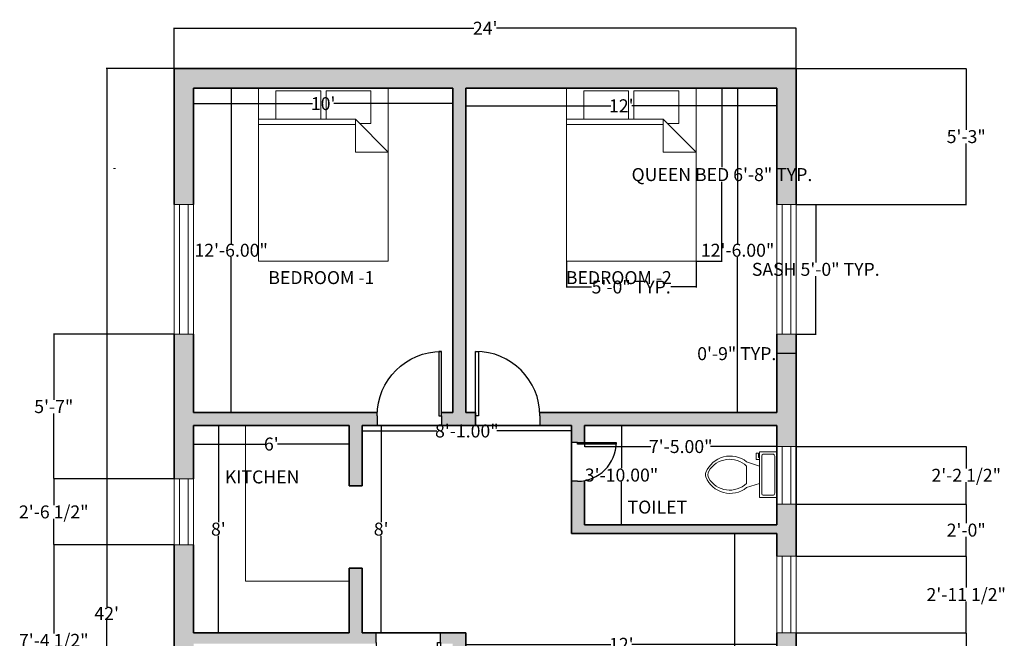
# Model space of a CAD drawing. Units: inches. Extents: x -54 to 402, y -41 to 548.
# Tile 2 of 2: x -53 to 402, y 261 to 548. Entities that reach past the tile are written whole.
import ezdxf

# ---------------------------------------------------------------- set-up
doc = ezdxf.new("R2010")
doc.units = ezdxf.units.IN
doc.header["$MEASUREMENT"] = 0
for name, color, linetype, lineweight in [('A-ANNO-DIMS', 2, 'Continuous', 18), ('A-AREA-IDEN', 7, 'Continuous', 25), ('A-DOOR', 4, 'Continuous', 25), ('A-FLOR-CASE', 8, 'Continuous', 18), ('A-FLOR-FIXT', 9, 'Continuous', 18), ('A-FURN', 8, 'Continuous', 18), ('A-GLAZ', 5, 'Continuous', 18), ('A-REFR', 8, 'Continuous', 13), ('A-WALL', 7, 'Continuous', 35)]:
    doc.layers.add(name, color=color, linetype=linetype, lineweight=lineweight)
doc.layers.add('A-WALL-PATT', color=18, linetype='Continuous', lineweight=13, true_color=0x000000)
doc.styles.get("Standard").update_dxf_attribs({"font": 'arial.ttf'})
doc.dimstyles.get("Standard").update_dxf_attribs({"dimtxt": 6, "dimasz": 0.18, "dimexe": 0.18, "dimexo": 0.0625, "dimgap": 0.09, "dimtad": 0, "dimtih": 1, "dimtoh": 1, "dimzin": 0, "dimdsep": 46, "dimlunit": 3, "dimtxsty": 'Standard', "dimcen": 0.09, "dimadec": 0, "dimazin": 0, "dimtfac": 1, "dimtofl": 0, "dimtmove": 0, "dimatfit": 3, "dimfxl": 1, "dimtolj": 1, "dimtzin": 0, "dimarcsym": 0})

# ---------------------------------------------------------------- blocks, each defined once
blk = doc.blocks.new('*U2')
for p, q in [((0, 0), (0, -6)), ((40, 0), (40, -6))]:
    blk.add_line(p, q)
blk.add_lwpolyline([(0, 0), (0, 40), (1.75, 40), (1.75, 0)], close=True)
blk.add_arc((0, 0), 40, 0, 90)
blk = doc.blocks.new('Bed - Queen')
for p, q in [((0, -80.00003), (0, 0)), ((0, 0), (59.99999, 0)), ((59.99999, 0), (59.99999, -80.00003)), ((7.99999, -1.2), (28.79998, -1.2)), ((7.99999, -14.4), (7.99999, -1.2)), ((28.79998, -1.2), (28.79998, -14.4)), ((31.19999, -1.2), (51.99999, -1.2)), ((31.19999, -14.4), (31.19999, -1.2)), ((51.99999, -1.2), (51.99999, -16.4)), ((0, -14.4), (44.8, -14.4)), ((44.8, -16.8), (0, -16.8)), ((59.99999, -29.6), (44.8, -14.4)), ((44.8, -14.4), (44.8, -29.6)), ((51.99999, -16.4), (46.79936, -16.4)), ((44.8, -29.6), (59.99999, -29.6)), ((59.99999, -80.00003), (0, -80.00003))]:
    blk.add_line(p, q)
blk = doc.blocks.new('*U5')
for p, q in [((9.5, -6), (9.5, -2)), ((-10, -8.5), (-8, -8.5)), ((-10, -9.5), (-10, -8.5)), ((-8, -8.5), (-8, -8)), ((-7, -8), (-7, -9.5)), ((-4, -8), (-6, -14)), ((4, -8), (6, -14)), ((-7, -9.5), (-10, -9.5)), ((4, -14), (-4, -14))]:
    blk.add_line(p, q)
blk.add_lwpolyline([(10.5, -8), (10.5, 0), (-10.5, 0), (-10.5, -8)], close=True)
for points in [[(-9.5, -2), (-9.5, -6)], [(8.5, -1), (-8.5, -1)], [(-8.5, -7), (8.5, -7)]]:
    blk.add_lwpolyline(points)
for centre, radius, start, end in [((-8.62, -1.88), 0.884, 81.8699, 188.1301), ((8.62, -1.88), 0.884, 351.8699, 98.1301), ((-8.62, -6.12), 0.884, 171.8699, 278.1301), ((8.62, -6.12), 0.884, 261.8699, 8.1301), ((3.52, -21.58), 12.17, 141.4691, 247.9714), ((4.2, -21.82), 11.33, 136.3677, 238.9468), ((-3.52, -21.58), 12.17, 292.0284, 38.5307), ((-4.2, -21.82), 11.33, 301.053, 43.6321), ((0, -27.88), 4, 245.7318, 294.2682), ((0, -29), 4, 254.8605, 285.1395)]:
    blk.add_arc(centre, radius, start, end)
blk = doc.blocks.new('*D6')
at = {"layer": 'A-ANNO-DIMS', "color": 0, "lineweight": -2, "transparency": 16777216}
for p, q in [((18.08, 524.92), (18.08, 543.75)), ((18.26, 543.57), (156.84, 543.57)), ((305.9, 543.57), (167.31, 543.57)), ((306.08, 524.92), (306.08, 543.75))]:
    blk.add_line(p, q, dxfattribs=at)
at = {"layer": 'A-ANNO-DIMS', "color": 0, "transparency": 16777216}
for points in [[(18.26, 543.6), (18.26, 543.54), (18.08, 543.57)], [(305.9, 543.6), (305.9, 543.54), (306.08, 543.57)]]:
    blk.add_solid(points, dxfattribs=at)
at = {"layer": 'Defpoints', "color": 0, "transparency": 16777216}
for p in [(306.08, 543.57), (18.08, 524.86), (306.08, 524.86)]:
    blk.add_point(p, dxfattribs=at)
at = {"layer": 'A-ANNO-DIMS', "color": 0, "transparency": 16777216, "insert": (162.08, 543.57), "char_height": 6, "attachment_point": 5}
blk.add_mtext("\\A1;24'", dxfattribs=at)
blk = doc.blocks.new('*D7')
at = {"layer": 'A-ANNO-DIMS', "color": 0, "lineweight": -2, "transparency": 16777216}
for p, q in [((18.01, 524.86), (-13.3, 524.86)), ((-13.12, 524.68), (-13.12, 275.96)), ((-13.12, 21.04), (-13.12, 269.76)), ((18.01, 20.86), (-13.3, 20.86))]:
    blk.add_line(p, q, dxfattribs=at)
at = {"layer": 'A-ANNO-DIMS', "color": 0, "transparency": 16777216}
for points in [[(-13.15, 524.68), (-13.09, 524.68), (-13.12, 524.86)], [(-13.15, 21.04), (-13.09, 21.04), (-13.12, 20.86)]]:
    blk.add_solid(points, dxfattribs=at)
at = {"layer": 'Defpoints', "color": 0, "transparency": 16777216}
for p in [(18.08, 524.86), (-13.12, 20.86), (18.08, 20.86)]:
    blk.add_point(p, dxfattribs=at)
at = {"layer": 'A-ANNO-DIMS', "color": 0, "transparency": 16777216, "insert": (-13.12, 272.86), "char_height": 6, "attachment_point": 5}
blk.add_mtext("\\A1;42'", dxfattribs=at)
blk = doc.blocks.new('*D15')
at = {"layer": 'A-ANNO-DIMS', "color": 0, "lineweight": -2, "transparency": 16777216}
for p, q in [((153.08, 263.8), (153.08, 258.38)), ((297.08, 263.8), (297.08, 258.38)), ((153.26, 258.56), (220.18, 258.56)), ((296.9, 258.56), (229.98, 258.56))]:
    blk.add_line(p, q, dxfattribs=at)
at = {"layer": 'A-ANNO-DIMS', "color": 0, "transparency": 16777216}
for points in [[(153.26, 258.59), (153.26, 258.53), (153.08, 258.56)], [(296.9, 258.59), (296.9, 258.53), (297.08, 258.56)]]:
    blk.add_solid(points, dxfattribs=at)
at = {"layer": 'Defpoints', "color": 0, "transparency": 16777216}
for p in [(153.08, 263.86), (297.08, 263.86), (297.08, 258.56)]:
    blk.add_point(p, dxfattribs=at)
at = {"layer": 'A-ANNO-DIMS', "color": 0, "transparency": 16777216, "insert": (225.08, 258.56), "char_height": 6, "attachment_point": 5}
blk.add_mtext("\\A1;12'", dxfattribs=at)
blk = doc.blocks.new('*D16')
at = {"layer": 'A-ANNO-DIMS', "color": 0, "lineweight": -2, "transparency": 16777216}
for p, q in [((297.01, 309.86), (277.33, 309.86)), ((277.51, 309.68), (277.51, 227.01)), ((277.51, 138.04), (277.51, 220.71)), ((297.01, 137.86), (277.33, 137.86))]:
    blk.add_line(p, q, dxfattribs=at)
at = {"layer": 'A-ANNO-DIMS', "color": 0, "transparency": 16777216}
for points in [[(277.48, 309.68), (277.54, 309.68), (277.51, 309.86)], [(277.48, 138.04), (277.54, 138.04), (277.51, 137.86)]]:
    blk.add_solid(points, dxfattribs=at)
at = {"layer": 'Defpoints', "color": 0, "transparency": 16777216}
for p in [(297.08, 309.86), (277.51, 137.86), (297.08, 137.86)]:
    blk.add_point(p, dxfattribs=at)
at = {"layer": 'A-ANNO-DIMS', "color": 0, "transparency": 16777216, "insert": (277.51, 223.86), "char_height": 6, "attachment_point": 5}
blk.add_mtext('\\A1;14\'-4.00"', dxfattribs=at)
blk = doc.blocks.new('*D17')
at = {"layer": 'A-ANNO-DIMS', "color": 0, "lineweight": -2, "transparency": 16777216}
for p, q in [((27.08, 359.8), (27.08, 351.03)), ((99.08, 359.8), (99.08, 351.03)), ((27.26, 351.21), (60.21, 351.21)), ((98.9, 351.21), (65.94, 351.21))]:
    blk.add_line(p, q, dxfattribs=at)
at = {"layer": 'A-ANNO-DIMS', "color": 0, "transparency": 16777216}
for points in [[(27.26, 351.24), (27.26, 351.18), (27.08, 351.21)], [(98.9, 351.24), (98.9, 351.18), (99.08, 351.21)]]:
    blk.add_solid(points, dxfattribs=at)
at = {"layer": 'Defpoints', "color": 0, "transparency": 16777216}
for p in [(27.08, 359.86), (99.08, 359.86), (99.08, 351.21)]:
    blk.add_point(p, dxfattribs=at)
at = {"layer": 'A-ANNO-DIMS', "color": 0, "transparency": 16777216, "insert": (63.08, 351.21), "char_height": 6, "attachment_point": 5}
blk.add_mtext("\\A1;6'", dxfattribs=at)
blk = doc.blocks.new('*D18')
at = {"layer": 'A-ANNO-DIMS', "color": 0, "lineweight": -2, "transparency": 16777216}
for p, q in [((32.47, 359.86), (38.75, 359.86)), ((38.57, 359.68), (38.57, 315.01)), ((38.57, 264.04), (38.57, 308.71)), ((32.47, 263.86), (38.75, 263.86))]:
    blk.add_line(p, q, dxfattribs=at)
at = {"layer": 'A-ANNO-DIMS', "color": 0, "transparency": 16777216}
for points in [[(38.54, 359.68), (38.6, 359.68), (38.57, 359.86)], [(38.54, 264.04), (38.6, 264.04), (38.57, 263.86)]]:
    blk.add_solid(points, dxfattribs=at)
at = {"layer": 'Defpoints', "color": 0, "transparency": 16777216}
for p in [(32.41, 359.86), (32.41, 263.86), (38.57, 263.86)]:
    blk.add_point(p, dxfattribs=at)
at = {"layer": 'A-ANNO-DIMS', "color": 0, "transparency": 16777216, "insert": (38.57, 311.86), "char_height": 6, "attachment_point": 5}
blk.add_mtext("\\A1;8'", dxfattribs=at)
blk = doc.blocks.new('*D19')
at = {"layer": 'A-ANNO-DIMS', "color": 0, "lineweight": -2, "transparency": 16777216}
for p, q in [((208.14, 359.86), (225.36, 359.86)), ((225.18, 359.68), (225.18, 340.02)), ((225.18, 314.04), (225.18, 333.71)), ((208.14, 313.86), (225.36, 313.86))]:
    blk.add_line(p, q, dxfattribs=at)
at = {"layer": 'A-ANNO-DIMS', "color": 0, "transparency": 16777216}
for points in [[(225.15, 359.68), (225.21, 359.68), (225.18, 359.86)], [(225.15, 314.04), (225.21, 314.04), (225.18, 313.86)]]:
    blk.add_solid(points, dxfattribs=at)
at = {"layer": 'Defpoints', "color": 0, "transparency": 16777216}
for p in [(208.08, 359.86), (208.08, 313.86), (225.18, 313.86)]:
    blk.add_point(p, dxfattribs=at)
at = {"layer": 'A-ANNO-DIMS', "color": 0, "transparency": 16777216, "insert": (225.18, 336.86), "char_height": 6, "attachment_point": 5}
blk.add_mtext('\\A1;3\'-10.00"', dxfattribs=at)
blk = doc.blocks.new('*D20')
at = {"layer": 'A-ANNO-DIMS', "color": 0, "lineweight": -2, "transparency": 16777216}
for p, q in [((208.08, 359.8), (208.08, 349.88)), ((297.08, 359.8), (297.08, 349.88)), ((208.26, 350.06), (238.71, 350.06)), ((296.9, 350.06), (266.44, 350.06))]:
    blk.add_line(p, q, dxfattribs=at)
at = {"layer": 'A-ANNO-DIMS', "color": 0, "transparency": 16777216}
for points in [[(208.26, 350.09), (208.26, 350.03), (208.08, 350.06)], [(296.9, 350.09), (296.9, 350.03), (297.08, 350.06)]]:
    blk.add_solid(points, dxfattribs=at)
at = {"layer": 'Defpoints', "color": 0, "transparency": 16777216}
for p in [(208.08, 359.86), (297.08, 359.86), (297.08, 350.06)]:
    blk.add_point(p, dxfattribs=at)
at = {"layer": 'A-ANNO-DIMS', "color": 0, "transparency": 16777216, "insert": (252.58, 350.06), "char_height": 6, "attachment_point": 5}
blk.add_mtext('\\A1;7\'-5.00"', dxfattribs=at)
blk = doc.blocks.new('*D21')
at = {"layer": 'A-ANNO-DIMS', "color": 0, "lineweight": -2, "transparency": 16777216}
for p, q in [((153.08, 515.8), (153.08, 507.5)), ((297.08, 515.8), (297.08, 507.5)), ((153.26, 507.68), (220.18, 507.68)), ((296.9, 507.68), (229.98, 507.68))]:
    blk.add_line(p, q, dxfattribs=at)
at = {"layer": 'A-ANNO-DIMS', "color": 0, "transparency": 16777216}
for points in [[(153.26, 507.71), (153.26, 507.65), (153.08, 507.68)], [(296.9, 507.71), (296.9, 507.65), (297.08, 507.68)]]:
    blk.add_solid(points, dxfattribs=at)
at = {"layer": 'Defpoints', "color": 0, "transparency": 16777216}
for p in [(153.08, 515.86), (297.08, 515.86), (297.08, 507.68)]:
    blk.add_point(p, dxfattribs=at)
at = {"layer": 'A-ANNO-DIMS', "color": 0, "transparency": 16777216, "insert": (225.08, 507.68), "char_height": 6, "attachment_point": 5}
blk.add_mtext("\\A1;12'", dxfattribs=at)
blk = doc.blocks.new('*D22')
at = {"layer": 'A-ANNO-DIMS', "color": 0, "lineweight": -2, "transparency": 16777216}
for p, q in [((297.01, 515.86), (278.73, 515.86)), ((278.91, 515.68), (278.91, 444.01)), ((278.91, 366.04), (278.91, 437.71)), ((297.01, 365.86), (278.73, 365.86))]:
    blk.add_line(p, q, dxfattribs=at)
at = {"layer": 'A-ANNO-DIMS', "color": 0, "transparency": 16777216}
for points in [[(278.88, 515.68), (278.94, 515.68), (278.91, 515.86)], [(278.88, 366.04), (278.94, 366.04), (278.91, 365.86)]]:
    blk.add_solid(points, dxfattribs=at)
at = {"layer": 'Defpoints', "color": 0, "transparency": 16777216}
for p in [(297.08, 515.86), (278.91, 365.86), (297.08, 365.86)]:
    blk.add_point(p, dxfattribs=at)
at = {"layer": 'A-ANNO-DIMS', "color": 0, "transparency": 16777216, "insert": (278.91, 440.86), "char_height": 6, "attachment_point": 5}
blk.add_mtext('\\A1;12\'-6.00"', dxfattribs=at)
blk = doc.blocks.new('*D23')
at = {"layer": 'A-ANNO-DIMS', "color": 0, "lineweight": -2, "transparency": 16777216}
for p, q in [((27.08, 515.8), (27.08, 508.5)), ((147.08, 515.8), (147.08, 508.5)), ((27.26, 508.68), (82.18, 508.68)), ((146.9, 508.68), (91.98, 508.68))]:
    blk.add_line(p, q, dxfattribs=at)
at = {"layer": 'A-ANNO-DIMS', "color": 0, "transparency": 16777216}
for points in [[(27.26, 508.71), (27.26, 508.65), (27.08, 508.68)], [(146.9, 508.71), (146.9, 508.65), (147.08, 508.68)]]:
    blk.add_solid(points, dxfattribs=at)
at = {"layer": 'Defpoints', "color": 0, "transparency": 16777216}
for p in [(27.08, 515.86), (147.08, 515.86), (147.08, 508.68)]:
    blk.add_point(p, dxfattribs=at)
at = {"layer": 'A-ANNO-DIMS', "color": 0, "transparency": 16777216, "insert": (87.08, 508.68), "char_height": 6, "attachment_point": 5}
blk.add_mtext("\\A1;10'", dxfattribs=at)
blk = doc.blocks.new('*D24')
at = {"layer": 'A-ANNO-DIMS', "color": 0, "lineweight": -2, "transparency": 16777216}
for p, q in [((46.31, 515.86), (44.31, 515.86)), ((44.49, 515.68), (44.49, 444.01)), ((44.49, 366.04), (44.49, 437.71)), ((46.31, 365.86), (44.31, 365.86))]:
    blk.add_line(p, q, dxfattribs=at)
at = {"layer": 'A-ANNO-DIMS', "color": 0, "transparency": 16777216}
for points in [[(44.46, 515.68), (44.52, 515.68), (44.49, 515.86)], [(44.46, 366.04), (44.52, 366.04), (44.49, 365.86)]]:
    blk.add_solid(points, dxfattribs=at)
at = {"layer": 'Defpoints', "color": 0, "transparency": 16777216}
for p in [(46.37, 515.86), (44.49, 365.86), (46.37, 365.86)]:
    blk.add_point(p, dxfattribs=at)
at = {"layer": 'A-ANNO-DIMS', "color": 0, "transparency": 16777216, "insert": (44.49, 440.86), "char_height": 6, "attachment_point": 5}
blk.add_mtext('\\A1;12\'-6.00"', dxfattribs=at)
blk = doc.blocks.new('*D25')
at = {"layer": 'A-ANNO-DIMS', "color": 0, "lineweight": -2, "transparency": 16777216}
for p, q in [((105.08, 359.8), (105.08, 357.08)), ((105.26, 357.26), (139.68, 357.26)), ((201.9, 357.26), (167.47, 357.26)), ((202.08, 359.8), (202.08, 357.08))]:
    blk.add_line(p, q, dxfattribs=at)
at = {"layer": 'A-ANNO-DIMS', "color": 0, "transparency": 16777216}
for points in [[(105.26, 357.29), (105.26, 357.23), (105.08, 357.26)], [(201.9, 357.29), (201.9, 357.23), (202.08, 357.26)]]:
    blk.add_solid(points, dxfattribs=at)
at = {"layer": 'Defpoints', "color": 0, "transparency": 16777216}
for p in [(105.08, 359.86), (202.08, 359.86), (202.08, 357.26)]:
    blk.add_point(p, dxfattribs=at)
at = {"layer": 'A-ANNO-DIMS', "color": 0, "transparency": 16777216, "insert": (153.58, 357.26), "char_height": 6, "attachment_point": 5}
blk.add_mtext('\\A1;8\'-1.00"', dxfattribs=at)
blk = doc.blocks.new('*D26')
at = {"layer": 'A-ANNO-DIMS', "color": 0, "lineweight": -2, "transparency": 16777216}
for p, q in [((105.14, 359.86), (114.09, 359.86)), ((113.91, 359.68), (113.91, 315.01)), ((113.91, 264.04), (113.91, 308.71)), ((105.14, 263.86), (114.09, 263.86))]:
    blk.add_line(p, q, dxfattribs=at)
at = {"layer": 'A-ANNO-DIMS', "color": 0, "transparency": 16777216}
for points in [[(113.88, 359.68), (113.94, 359.68), (113.91, 359.86)], [(113.88, 264.04), (113.94, 264.04), (113.91, 263.86)]]:
    blk.add_solid(points, dxfattribs=at)
at = {"layer": 'Defpoints', "color": 0, "transparency": 16777216}
for p in [(105.08, 359.86), (105.08, 263.86), (113.91, 263.86)]:
    blk.add_point(p, dxfattribs=at)
at = {"layer": 'A-ANNO-DIMS', "color": 0, "transparency": 16777216, "insert": (113.91, 311.86), "char_height": 6, "attachment_point": 5}
blk.add_mtext("\\A1;8'", dxfattribs=at)
blk = doc.blocks.new('WIN-60IN-SASH')
for p, q in [((0, 60), (9, 60)), ((0, 0), (9, 0))]:
    blk.add_line(p, q)
for points in [[(2.5, 60), (2.5, 0)], [(6.5, 60), (6.5, 0)]]:
    blk.add_lwpolyline(points)
blk = doc.blocks.new('*D28')
at = {"layer": 'A-ANNO-DIMS', "color": 0, "lineweight": -2, "transparency": 16777216}
for p, q in [((259.73, 515.86), (271.84, 515.86)), ((271.66, 515.68), (271.66, 479.24)), ((271.66, 436.04), (271.66, 472.48)), ((259.73, 435.86), (271.84, 435.86))]:
    blk.add_line(p, q, dxfattribs=at)
at = {"layer": 'A-ANNO-DIMS', "color": 0, "transparency": 16777216}
for points in [[(271.63, 515.68), (271.69, 515.68), (271.66, 515.86)], [(271.63, 436.04), (271.69, 436.04), (271.66, 435.86)]]:
    blk.add_solid(points, dxfattribs=at)
at = {"layer": 'Defpoints', "color": 0, "transparency": 16777216}
for p in [(259.66, 515.86), (271.66, 515.86), (259.66, 435.86)]:
    blk.add_point(p, dxfattribs=at)
at = {"layer": 'A-ANNO-DIMS', "color": 0, "transparency": 16777216, "insert": (271.66, 475.86), "char_height": 6, "attachment_point": 5}
blk.add_mtext('\\A1;QUEEN BED 6\'-8" TYP.', dxfattribs=at)
blk = doc.blocks.new('*D29')
at = {"layer": 'A-ANNO-DIMS', "color": 0, "lineweight": -2, "transparency": 16777216}
for p, q in [((199.66, 435.8), (199.66, 423.68)), ((259.66, 435.8), (259.66, 423.68)), ((199.84, 423.86), (211.29, 423.86)), ((259.48, 423.86), (248.04, 423.86))]:
    blk.add_line(p, q, dxfattribs=at)
at = {"layer": 'A-ANNO-DIMS', "color": 0, "transparency": 16777216}
for points in [[(199.84, 423.89), (199.84, 423.83), (199.66, 423.86)], [(259.48, 423.89), (259.48, 423.83), (259.66, 423.86)]]:
    blk.add_solid(points, dxfattribs=at)
at = {"layer": 'Defpoints', "color": 0, "transparency": 16777216}
for p in [(199.66, 435.86), (259.66, 435.86), (259.66, 423.86)]:
    blk.add_point(p, dxfattribs=at)
at = {"layer": 'A-ANNO-DIMS', "color": 0, "transparency": 16777216, "insert": (229.66, 423.86), "char_height": 6, "attachment_point": 5}
blk.add_mtext('\\A1;5\'-0" TYP.', dxfattribs=at)
blk = doc.blocks.new('*D30')
at = {"layer": 'A-ANNO-DIMS', "color": 0, "lineweight": -2, "transparency": 16777216}
for p, q in [((306.14, 462.03), (315.26, 462.03)), ((315.08, 461.85), (315.08, 435.22)), ((315.08, 402.21), (315.08, 428.84)), ((306.14, 402.03), (315.26, 402.03))]:
    blk.add_line(p, q, dxfattribs=at)
at = {"layer": 'A-ANNO-DIMS', "color": 0, "transparency": 16777216}
for points in [[(315.05, 461.85), (315.11, 461.85), (315.08, 462.03)], [(315.05, 402.21), (315.11, 402.21), (315.08, 402.03)]]:
    blk.add_solid(points, dxfattribs=at)
at = {"layer": 'Defpoints', "color": 0, "transparency": 16777216}
for p in [(306.08, 462.03), (306.08, 402.03), (315.08, 402.03)]:
    blk.add_point(p, dxfattribs=at)
at = {"layer": 'A-ANNO-DIMS', "color": 0, "transparency": 16777216, "insert": (315.08, 432.03), "char_height": 6, "attachment_point": 5}
blk.add_mtext('\\A1;SASH 5\'-0" TYP.', dxfattribs=at)
blk = doc.blocks.new('*D31')
at = {"layer": 'A-ANNO-DIMS', "color": 0, "lineweight": -2, "transparency": 16777216}
for p, q in [((297.08, 401.97), (297.08, 392.85)), ((306.08, 401.97), (306.08, 392.85)), ((297.08, 393.03), (296.9, 393.03)), ((305.9, 393.03), (297.26, 393.03))]:
    blk.add_line(p, q, dxfattribs=at)
at = {"layer": 'A-ANNO-DIMS', "color": 0, "transparency": 16777216}
for points in [[(297.26, 393.06), (297.26, 393), (297.08, 393.03)], [(305.9, 393.06), (305.9, 393), (306.08, 393.03)]]:
    blk.add_solid(points, dxfattribs=at)
at = {"layer": 'Defpoints', "color": 0, "transparency": 16777216}
for p in [(297.08, 402.03), (306.08, 402.03), (297.08, 393.03)]:
    blk.add_point(p, dxfattribs=at)
at = {"layer": 'A-ANNO-DIMS', "color": 0, "transparency": 16777216, "insert": (278.52, 393.03), "char_height": 6, "attachment_point": 5}
blk.add_mtext('\\A1;0\'-9" TYP.', dxfattribs=at)
blk = doc.blocks.new('*D36')
at = {"layer": 'A-ANNO-DIMS', "color": 0, "lineweight": -2, "transparency": 16777216}
for p, q in [((18.01, 304.58), (-37.79, 304.58)), ((-37.61, 304.4), (-37.61, 263.59)), ((-37.61, 216.4), (-37.61, 257.21)), ((18.01, 216.22), (-37.79, 216.22))]:
    blk.add_line(p, q, dxfattribs=at)
at = {"layer": 'A-ANNO-DIMS', "color": 0, "transparency": 16777216}
for points in [[(-37.64, 304.4), (-37.58, 304.4), (-37.61, 304.58)], [(-37.64, 216.4), (-37.58, 216.4), (-37.61, 216.22)]]:
    blk.add_solid(points, dxfattribs=at)
at = {"layer": 'Defpoints', "color": 0, "transparency": 16777216}
for p in [(-37.61, 304.58), (18.08, 304.58), (18.08, 216.22)]:
    blk.add_point(p, dxfattribs=at)
at = {"layer": 'A-ANNO-DIMS', "color": 0, "transparency": 16777216, "insert": (-37.61, 260.4), "char_height": 6, "attachment_point": 5}
blk.add_mtext('\\A1;7\'-4 1/2"', dxfattribs=at)
blk = doc.blocks.new('*D37')
at = {"layer": 'A-ANNO-DIMS', "color": 0, "lineweight": -2, "transparency": 16777216}
for p, q in [((18.01, 335.06), (-37.79, 335.06)), ((-37.61, 334.88), (-37.61, 323.01)), ((-37.61, 304.76), (-37.61, 316.63)), ((18.01, 304.58), (-37.79, 304.58))]:
    blk.add_line(p, q, dxfattribs=at)
at = {"layer": 'A-ANNO-DIMS', "color": 0, "transparency": 16777216}
for points in [[(-37.64, 334.88), (-37.58, 334.88), (-37.61, 335.06)], [(-37.64, 304.76), (-37.58, 304.76), (-37.61, 304.58)]]:
    blk.add_solid(points, dxfattribs=at)
at = {"layer": 'Defpoints', "color": 0, "transparency": 16777216}
for p in [(-37.61, 335.06), (18.08, 335.06), (18.08, 304.58)]:
    blk.add_point(p, dxfattribs=at)
at = {"layer": 'A-ANNO-DIMS', "color": 0, "transparency": 16777216, "insert": (-37.61, 319.82), "char_height": 6, "attachment_point": 5}
blk.add_mtext('\\A1;2\'-6 1/2"', dxfattribs=at)
blk = doc.blocks.new('*D38')
at = {"layer": 'A-ANNO-DIMS', "color": 0, "lineweight": -2, "transparency": 16777216}
for p, q in [((18.01, 402.03), (-37.79, 402.03)), ((-37.61, 401.85), (-37.61, 371.69)), ((-37.61, 335.24), (-37.61, 365.4)), ((18.01, 335.06), (-37.79, 335.06))]:
    blk.add_line(p, q, dxfattribs=at)
at = {"layer": 'A-ANNO-DIMS', "color": 0, "transparency": 16777216}
for points in [[(-37.64, 401.85), (-37.58, 401.85), (-37.61, 402.03)], [(-37.64, 335.24), (-37.58, 335.24), (-37.61, 335.06)]]:
    blk.add_solid(points, dxfattribs=at)
at = {"layer": 'Defpoints', "color": 0, "transparency": 16777216}
for p in [(-37.61, 402.03), (18.08, 402.03), (18.08, 335.06)]:
    blk.add_point(p, dxfattribs=at)
at = {"layer": 'A-ANNO-DIMS', "color": 0, "transparency": 16777216, "insert": (-37.61, 368.54), "char_height": 6, "attachment_point": 5}
blk.add_mtext('\\A1;5\'-7"', dxfattribs=at)
blk = doc.blocks.new('*D43')
at = {"layer": 'A-ANNO-DIMS', "color": 0, "lineweight": -2, "transparency": 16777216}
for p, q in [((306.14, 263.86), (384.91, 263.86)), ((384.73, 263.68), (384.73, 232.29)), ((384.73, 194.51), (384.73, 225.91)), ((306.14, 194.33), (384.91, 194.33))]:
    blk.add_line(p, q, dxfattribs=at)
at = {"layer": 'A-ANNO-DIMS', "color": 0, "transparency": 16777216}
for points in [[(384.7, 263.68), (384.76, 263.68), (384.73, 263.86)], [(384.7, 194.51), (384.76, 194.51), (384.73, 194.33)]]:
    blk.add_solid(points, dxfattribs=at)
at = {"layer": 'Defpoints', "color": 0, "transparency": 16777216}
for p in [(306.08, 263.86), (384.73, 263.86), (306.08, 194.33)]:
    blk.add_point(p, dxfattribs=at)
at = {"layer": 'A-ANNO-DIMS', "color": 0, "transparency": 16777216, "insert": (384.73, 229.1), "char_height": 6, "attachment_point": 5}
blk.add_mtext('\\A1;5\'-9 1/2"', dxfattribs=at)
blk = doc.blocks.new('*D44')
at = {"layer": 'A-ANNO-DIMS', "color": 0, "lineweight": -2, "transparency": 16777216}
for p, q in [((306.14, 299.34), (384.91, 299.34)), ((384.73, 299.16), (384.73, 284.79)), ((384.73, 264.04), (384.73, 278.41)), ((306.14, 263.86), (384.91, 263.86))]:
    blk.add_line(p, q, dxfattribs=at)
at = {"layer": 'A-ANNO-DIMS', "color": 0, "transparency": 16777216}
for points in [[(384.7, 299.16), (384.76, 299.16), (384.73, 299.34)], [(384.7, 264.04), (384.76, 264.04), (384.73, 263.86)]]:
    blk.add_solid(points, dxfattribs=at)
at = {"layer": 'Defpoints', "color": 0, "transparency": 16777216}
for p in [(306.08, 299.34), (384.73, 299.34), (306.08, 263.86)]:
    blk.add_point(p, dxfattribs=at)
at = {"layer": 'A-ANNO-DIMS', "color": 0, "transparency": 16777216, "insert": (384.73, 281.6), "char_height": 6, "attachment_point": 5}
blk.add_mtext('\\A1;2\'-11 1/2"', dxfattribs=at)
blk = doc.blocks.new('*D45')
at = {"layer": 'A-ANNO-DIMS', "color": 0, "lineweight": -2, "transparency": 16777216}
for p, q in [((306.14, 323.46), (384.91, 323.46)), ((384.73, 323.28), (384.73, 314.55)), ((384.73, 299.52), (384.73, 308.24)), ((306.14, 299.34), (384.91, 299.34))]:
    blk.add_line(p, q, dxfattribs=at)
at = {"layer": 'A-ANNO-DIMS', "color": 0, "transparency": 16777216}
for points in [[(384.7, 323.28), (384.76, 323.28), (384.73, 323.46)], [(384.7, 299.52), (384.76, 299.52), (384.73, 299.34)]]:
    blk.add_solid(points, dxfattribs=at)
at = {"layer": 'Defpoints', "color": 0, "transparency": 16777216}
for p in [(306.08, 323.46), (384.73, 323.46), (306.08, 299.34)]:
    blk.add_point(p, dxfattribs=at)
at = {"layer": 'A-ANNO-DIMS', "color": 0, "transparency": 16777216, "insert": (384.73, 311.4), "char_height": 6, "attachment_point": 5}
blk.add_mtext('\\A1;2\'-0"', dxfattribs=at)
blk = doc.blocks.new('*D46')
at = {"layer": 'A-ANNO-DIMS', "color": 0, "lineweight": -2, "transparency": 16777216}
for p, q in [((306.14, 350.06), (384.91, 350.06)), ((384.73, 349.88), (384.73, 339.95)), ((384.73, 323.64), (384.73, 333.57)), ((306.14, 323.46), (384.91, 323.46))]:
    blk.add_line(p, q, dxfattribs=at)
at = {"layer": 'A-ANNO-DIMS', "color": 0, "transparency": 16777216}
for points in [[(384.7, 349.88), (384.76, 349.88), (384.73, 350.06)], [(384.7, 323.64), (384.76, 323.64), (384.73, 323.46)]]:
    blk.add_solid(points, dxfattribs=at)
at = {"layer": 'Defpoints', "color": 0, "transparency": 16777216}
for p in [(306.08, 350.06), (384.73, 350.06), (306.08, 323.46)]:
    blk.add_point(p, dxfattribs=at)
at = {"layer": 'A-ANNO-DIMS', "color": 0, "transparency": 16777216, "insert": (384.73, 336.76), "char_height": 6, "attachment_point": 5}
blk.add_mtext('\\A1;2\'-2 1/2"', dxfattribs=at)
blk = doc.blocks.new('*D47')
at = {"layer": 'A-ANNO-DIMS', "color": 0, "lineweight": -2, "transparency": 16777216}
for p, q in [((306.14, 524.86), (384.91, 524.86)), ((384.73, 524.68), (384.73, 496.6)), ((384.73, 462.21), (384.73, 490.29)), ((306.14, 462.03), (384.91, 462.03))]:
    blk.add_line(p, q, dxfattribs=at)
at = {"layer": 'A-ANNO-DIMS', "color": 0, "transparency": 16777216}
for points in [[(384.7, 524.68), (384.76, 524.68), (384.73, 524.86)], [(384.7, 462.21), (384.76, 462.21), (384.73, 462.03)]]:
    blk.add_solid(points, dxfattribs=at)
at = {"layer": 'Defpoints', "color": 0, "transparency": 16777216}
for p in [(306.08, 524.86), (384.73, 524.86), (306.08, 462.03)]:
    blk.add_point(p, dxfattribs=at)
at = {"layer": 'A-ANNO-DIMS', "color": 0, "transparency": 16777216, "insert": (384.73, 493.44), "char_height": 6, "attachment_point": 5}
blk.add_mtext('\\A1;5\'-3"', dxfattribs=at)

msp = doc.modelspace()

# ---------------------------------------------------------------- hatches: boundary and pattern name
at = {"layer": 'A-WALL-PATT'}
h = msp.add_hatch(color=256, dxfattribs=at)
h.dxf.hatch_style = 1
h.paths.add_polyline_path([(306.077, 402.028), (297.077, 402.028), (297.077, 365.861), (187.375, 365.861, -0.0129064), (187.414, 364.326), (187.414, 359.861), (202.077, 359.861), (202.077, 351.989), (204.773, 351.989), (208.077, 351.989), (208.077, 359.861), (297.077, 359.861), (297.077, 350.063), (306.077, 350.063)])
h.paths.add_polyline_path([(306.077, 323.455), (297.077, 323.455), (297.077, 313.861), (208.077, 313.861), (208.077, 334.328, -0.0462821), (204.773, 334.022), (202.077, 334.022), (202.077, 309.861), (297.077, 309.861), (297.077, 299.338), (306.077, 299.338)])
h.paths.add_polyline_path([(153.077, 515.861), (297.077, 515.861), (297.077, 462.028), (306.077, 462.028), (306.077, 524.861), (18.077, 524.861), (18.077, 462.028), (27.077, 462.028), (27.077, 515.861), (147.077, 515.861), (147.077, 365.861), (141.864, 365.861), (141.864, 364.326), (141.864, 359.861), (157.652, 359.861), (157.652, 364.326), (157.652, 365.861), (153.077, 365.861)])
h.paths.add_polyline_path([(137.933, 351.035), (169.275, 351.035), (169.275, 363.399), (137.933, 363.399)], flags=9)
h = msp.add_hatch(color=256, dxfattribs=at)
h.dxf.hatch_style = 1
h.paths.add_polyline_path([(306.077, 149.429), (297.077, 149.429), (297.077, 137.861), (188.036, 137.861, -0.0129064), (188.075, 136.326), (188.075, 131.861), (297.077, 131.861), (297.077, 83.839), (306.077, 83.839)])
h.paths.add_polyline_path([(306.077, 263.861), (297.077, 263.861), (297.077, 194.333), (306.077, 194.333)])
h.paths.add_polyline_path([(306.077, 44.446), (297.077, 44.446), (297.077, 29.861), (203.639, 29.861, -0.015458), (203.72, 27.236), (203.72, 20.861), (306.077, 20.861)])
h.paths.add_polyline_path([(55.334, 29.861), (27.077, 29.861), (27.077, 60.781), (18.077, 60.781), (18.077, 20.861), (55.334, 20.861)])
h.paths.add_polyline_path([(161.225, 27.236), (161.225, 29.861), (153.077, 29.861), (153.077, 95.263), (148.613, 95.263, -0.0129064), (147.077, 95.303), (147.077, 29.861), (101.039, 29.861), (101.039, 20.861), (161.225, 20.861)])
h.paths.add_polyline_path([(158.313, 136.326), (158.313, 137.861), (153.077, 137.861), (153.077, 263.861), (141.33, 263.861), (141.33, 259.397), (141.33, 258.861), (147.077, 258.861), (147.077, 137.861), (27.077, 137.861), (27.077, 167.529), (18.077, 167.529), (18.077, 101.294), (27.077, 101.294), (27.077, 131.861), (147.077, 131.861), (147.077, 125.025), (148.613, 125.025), (153.077, 125.025), (153.077, 131.861), (158.313, 131.861)])
h.paths.add_polyline_path([(111.568, 263.861), (105.077, 263.861), (105.077, 293.745), (99.077, 293.745), (99.077, 263.861), (27.077, 263.861), (27.077, 304.579), (18.077, 304.579), (18.077, 216.221), (27.077, 216.221), (27.077, 258.861), (111.573, 258.861, -0.0045002), (111.568, 259.397)])
h.paths.add_polyline_path([(112.102, 364.326, -0.0129064), (112.142, 365.861), (27.077, 365.861), (27.077, 402.028), (18.077, 402.028), (18.077, 335.061), (27.077, 335.061), (27.077, 359.861), (99.077, 359.861), (99.077, 331.859), (105.077, 331.859), (105.077, 359.861), (112.102, 359.861)])

# ---------------------------------------------------------------- linework, layer by layer
at = {"layer": 'A-FLOR-CASE'}
for points in [[(51.077, 359.861), (51.077, 287.861)], [(99.077, 287.861), (51.077, 287.861)]]:
    msp.add_lwpolyline(points, dxfattribs=at)
at = {"layer": 'A-GLAZ'}
for p, q in [((297.077, 350.063), (306.077, 350.063)), ((27.077, 335.061), (18.077, 335.061)), ((297.077, 323.455), (306.077, 323.455)), ((18.077, 304.579), (27.077, 304.579)), ((297.077, 299.338), (306.077, 299.338)), ((297.077, 263.861), (306.077, 263.861))]:
    msp.add_line(p, q, dxfattribs=at)
for points in [[(18.077, 462.028), (27.077, 462.028), (27.077, 402.028), (18.077, 402.028)], [(297.077, 462.028), (306.077, 462.028), (306.077, 402.028), (297.077, 402.028)], [(18.077, 335.061), (27.077, 335.061), (27.077, 304.579), (18.077, 304.579)], [(297.077, 299.338), (306.077, 299.338), (306.077, 263.861), (297.077, 263.861)]]:
    msp.add_lwpolyline(points, close=True, dxfattribs=at)
for points in [[(299.577, 323.455), (299.577, 350.063)], [(303.577, 323.455), (303.577, 350.063)], [(20.577, 335.061), (20.577, 304.579)], [(24.577, 335.061), (24.577, 304.579)], [(299.577, 263.861), (299.577, 299.338)], [(303.577, 263.861), (303.577, 299.338)]]:
    msp.add_lwpolyline(points, dxfattribs=at)
at = {"layer": 'A-REFR'}
msp.add_lwpolyline([(-9.039, 478.625), (-9.959, 478.625), (-9.959, 478.625), (-9.039, 478.625)], close=True, dxfattribs=at)
at = {"layer": 'A-WALL'}
for p, q in [((142.296, 365.861), (141.864, 365.861)), ((147.077, 365.861), (142.296, 365.861)), ((142.296, 365.861), (142.296, 365.861)), ((157.652, 365.861), (157.652, 359.861)), ((208.077, 313.861), (208.077, 334.328)), ((99.077, 331.859), (105.077, 331.859)), ((99.077, 293.745), (105.077, 293.745))]:
    msp.add_line(p, q, dxfattribs=at)
for points in [[(306.077, 462.028), (306.077, 524.861), (18.077, 524.861), (18.077, 462.028)], [(27.077, 515.861), (27.077, 462.028)], [(147.077, 515.861), (27.077, 515.861)], [(147.077, 515.861), (147.077, 365.861)], [(297.077, 515.861), (153.077, 515.861)], [(153.077, 365.861), (153.077, 515.861)], [(297.077, 462.028), (297.077, 515.861)], [(18.077, 402.028), (18.077, 335.061)], [(27.077, 402.028), (27.077, 365.861)], [(297.077, 365.861), (297.077, 402.028)], [(306.077, 299.338), (306.077, 402.028)], [(112.142, 365.861), (27.077, 365.861)], [(147.077, 365.861), (141.864, 365.861)], [(157.652, 365.861), (153.077, 365.861)], [(297.077, 365.861), (187.375, 365.861)], [(27.077, 359.861), (27.077, 335.061)], [(99.077, 359.861), (27.077, 359.861)], [(99.077, 359.861), (99.077, 331.859)], [(105.077, 359.861), (105.077, 331.859)], [(202.077, 359.861), (105.077, 359.861)], [(202.077, 359.861), (202.077, 309.861)], [(297.077, 359.861), (208.077, 359.861)], [(208.077, 351.203), (208.077, 359.861)], [(297.077, 313.861), (297.077, 359.861)], [(297.077, 313.861), (208.077, 313.861)], [(202.077, 309.861), (297.077, 309.861)], [(297.077, 299.338), (297.077, 309.861)], [(297.077, 299.338), (297.077, 307.861)], [(18.077, 304.579), (18.077, 216.221)], [(27.077, 304.579), (27.077, 263.861)], [(99.077, 293.745), (99.077, 263.861)], [(105.077, 293.745), (105.077, 263.861)], [(99.077, 263.861), (27.077, 263.861)], [(153.077, 263.861), (105.077, 263.861)], [(153.077, 137.861), (153.077, 263.861)], [(297.077, 194.333), (297.077, 263.861)], [(306.077, 194.333), (306.077, 263.861)]]:
    msp.add_lwpolyline(points, dxfattribs=at)

# ---------------------------------------------------------------- block references
at = {"layer": 'A-DOOR', "yscale": 0.7440482998037414, "zscale": 0.7440482998037414}
for p, xscale in [((141.864, 364.326), -0.7440482998037414), ((157.652, 364.326), 0.7440482998037414)]:
    msp.add_blockref('*U2', p, dxfattribs=dict(at, xscale=xscale))
at = {"layer": 'A-DOOR'}
for p, xscale, yscale, zscale, rotation in [((204.773, 351.989), 0.449178302334471, 0.449178302334471, 0.449178302334471, 270), ((141.33, 259.397), 0.7440482998037414, 0.7440482998037414, 0.7440482998037414, 180)]:
    msp.add_blockref('*U2', p, dxfattribs=dict(at, xscale=xscale, yscale=yscale, zscale=zscale, rotation=rotation))
at = {"layer": 'A-FLOR-FIXT', "rotation": 270}
msp.add_blockref('*U5', (297.077, 337.038), dxfattribs=at)
at = {"layer": 'A-FURN'}
for p in [(57.207, 515.861), (199.664, 515.861)]:
    msp.add_blockref('Bed - Queen', p, dxfattribs=at)
at = {"layer": 'A-GLAZ'}
msp.add_blockref('WIN-60IN-SASH', (18.077, 402.028), dxfattribs=at)
at = {"layer": 'A-GLAZ', "rotation": 180}
msp.add_blockref('WIN-60IN-SASH', (306.077, 462.028), dxfattribs=at)

# ---------------------------------------------------------------- texts
at = {"layer": 'A-AREA-IDEN', "char_height": 6, "attachment_point": 1}
for s, insert in [('BEDROOM -1', (61.717, 431.197)), ('BEDROOM -2', (199.413, 431.197)), ('KITCHEN', (41.575, 339.012)), ('TOILET', (227.991, 325.052))]:
    msp.add_mtext_dynamic_manual_height_columns(s, width=186.62834, gutter_width=1, heights=[0], dxfattribs=dict(at, insert=insert))

# ---------------------------------------------------------------- dimensions: what is measured, and where the dimension line sits
at = {"layer": 'A-ANNO-DIMS'}
for base, p1, p2, picture, middle in [((306.077, 543.565), (18.077, 524.861), (306.077, 524.861), '*D6', (162.077, 543.565)), ((147.077, 508.678), (27.077, 515.861), (147.077, 515.861), '*D23', (87.077, 508.678)), ((297.077, 507.678), (153.077, 515.861), (297.077, 515.861), '*D21', (225.077, 507.678)), ((202.077, 357.26), (105.077, 359.861), (202.077, 359.861), '*D25', (153.577, 357.26)), ((99.077, 351.21), (27.077, 359.861), (99.077, 359.861), '*D17', (63.077, 351.21)), ((297.077, 350.063), (208.077, 359.861), (297.077, 359.861), '*D20', (252.577, 350.063)), ((297.077, 258.564), (153.077, 263.861), (297.077, 263.861), '*D15', (225.077, 258.564))]:
    dim = msp.add_linear_dim(base=base, p1=p1, p2=p2, dimstyle='Standard', override={"dimclrd": 0, "dimclre": 0, "dimclrt": 0}, dxfattribs=at)
    dim.commit()
    dim.dimension.update_dxf_attribs({"geometry": picture, "text_midpoint": middle})
for base, p1, p2, override, picture, middle in [((-13.116, 20.861), (18.077, 524.861), (18.077, 20.861), {"dimclrd": 0, "dimclre": 0, "dimclrt": 0}, '*D7', (-13.116, 272.861)), ((384.727, 524.861), (306.077, 462.028), (306.077, 524.861), {"dimdec": 1, "dimlfac": 1, "dimrnd": 0, "dimzin": 1, "dimdsep": 46, "dimlunit": 4, "dimfrac": 2}, '*D47', (384.727, 493.444)), ((44.491, 365.861), (46.37, 515.861), (46.37, 365.861), {"dimclrd": 0, "dimclre": 0, "dimclrt": 0}, '*D24', (44.491, 440.861)), ((278.907, 365.861), (297.077, 515.861), (297.077, 365.861), {"dimclrd": 0, "dimclre": 0, "dimclrt": 0}, '*D22', (278.907, 440.861)), ((-37.609, 402.028), (18.077, 335.061), (18.077, 402.028), {"dimdec": 1, "dimlfac": 1, "dimrnd": 0, "dimzin": 1, "dimdsep": 46, "dimlunit": 4, "dimfrac": 2}, '*D38', (-37.609, 368.544)), ((38.568, 263.861), (32.406, 359.861), (32.406, 263.861), {"dimclrd": 0, "dimclre": 0, "dimclrt": 0}, '*D18', (38.568, 311.861)), ((113.913, 263.861), (105.077, 359.861), (105.077, 263.861), {"dimclrd": 0, "dimclre": 0, "dimclrt": 0}, '*D26', (113.913, 311.861)), ((225.183, 313.861), (208.077, 359.861), (208.077, 313.861), {"dimclrd": 0, "dimclre": 0, "dimclrt": 0}, '*D19', (225.183, 336.861)), ((384.727, 350.063), (306.077, 323.455), (306.077, 350.063), {"dimdec": 1, "dimlfac": 1, "dimrnd": 0, "dimzin": 1, "dimdsep": 46, "dimlunit": 4, "dimfrac": 2}, '*D46', (384.727, 336.759)), ((-37.609, 335.061), (18.077, 304.579), (18.077, 335.061), {"dimdec": 1, "dimlfac": 1, "dimrnd": 0, "dimzin": 1, "dimdsep": 46, "dimlunit": 4, "dimfrac": 2}, '*D37', (-37.609, 319.82)), ((384.727, 323.455), (306.077, 299.338), (306.077, 323.455), {"dimdec": 1, "dimlfac": 1, "dimrnd": 0, "dimzin": 1, "dimdsep": 46, "dimlunit": 4, "dimfrac": 2}, '*D45', (384.727, 311.397)), ((277.507, 137.861), (297.077, 309.861), (297.077, 137.861), {"dimclrd": 0, "dimclre": 0, "dimclrt": 0}, '*D16', (277.507, 223.861)), ((-37.609, 304.579), (18.077, 216.221), (18.077, 304.579), {"dimdec": 1, "dimlfac": 1, "dimrnd": 0, "dimzin": 1, "dimdsep": 46, "dimlunit": 4, "dimfrac": 2}, '*D36', (-37.609, 260.4)), ((384.727, 299.338), (306.077, 263.861), (306.077, 299.338), {"dimdec": 1, "dimlfac": 1, "dimrnd": 0, "dimzin": 1, "dimdsep": 46, "dimlunit": 4, "dimfrac": 2}, '*D44', (384.727, 281.6)), ((384.727, 263.861), (306.077, 194.333), (306.077, 263.861), {"dimdec": 1, "dimlfac": 1, "dimrnd": 0, "dimzin": 1, "dimdsep": 46, "dimlunit": 4, "dimfrac": 2}, '*D43', (384.727, 229.097))]:
    dim = msp.add_linear_dim(base=base, p1=p1, p2=p2, angle=90, dimstyle='Standard', override=override, dxfattribs=at)
    dim.commit()
    dim.dimension.update_dxf_attribs({"geometry": picture, "text_midpoint": middle})
for base, p1, p2, angle, text, picture, middle in [((271.664, 515.861), (259.664, 435.861), (259.664, 515.861), 90, 'QUEEN BED <> TYP.', '*D28', (271.664, 475.861)), ((315.077, 402.028), (306.077, 462.028), (306.077, 402.028), 270, 'SASH <> TYP.', '*D30', (315.077, 432.028)), ((297.077, 393.028), (306.077, 402.028), (297.077, 402.028), 180, '<> TYP.', '*D31', (278.521, 393.028))]:
    dim = msp.add_linear_dim(base=base, p1=p1, p2=p2, angle=angle, text=text, dimstyle='Standard', override={"dimdec": 1, "dimlfac": 1, "dimrnd": 0, "dimzin": 1, "dimdsep": 46, "dimlunit": 4, "dimfrac": 2}, dxfattribs=at)
    dim.commit()
    dim.dimension.update_dxf_attribs({"geometry": picture, "text_midpoint": middle})
dim = msp.add_linear_dim(base=(259.664, 423.861), p1=(199.664, 435.861), p2=(259.664, 435.861), text='<> TYP.', dimstyle='Standard', override={"dimdec": 1, "dimlfac": 1, "dimrnd": 0, "dimzin": 1, "dimdsep": 46, "dimlunit": 4, "dimfrac": 2}, dxfattribs=at)
dim.commit()
dim.dimension.update_dxf_attribs({"geometry": '*D29', "text_midpoint": (229.664, 423.861)})

doc.saveas('drawing.dxf')
